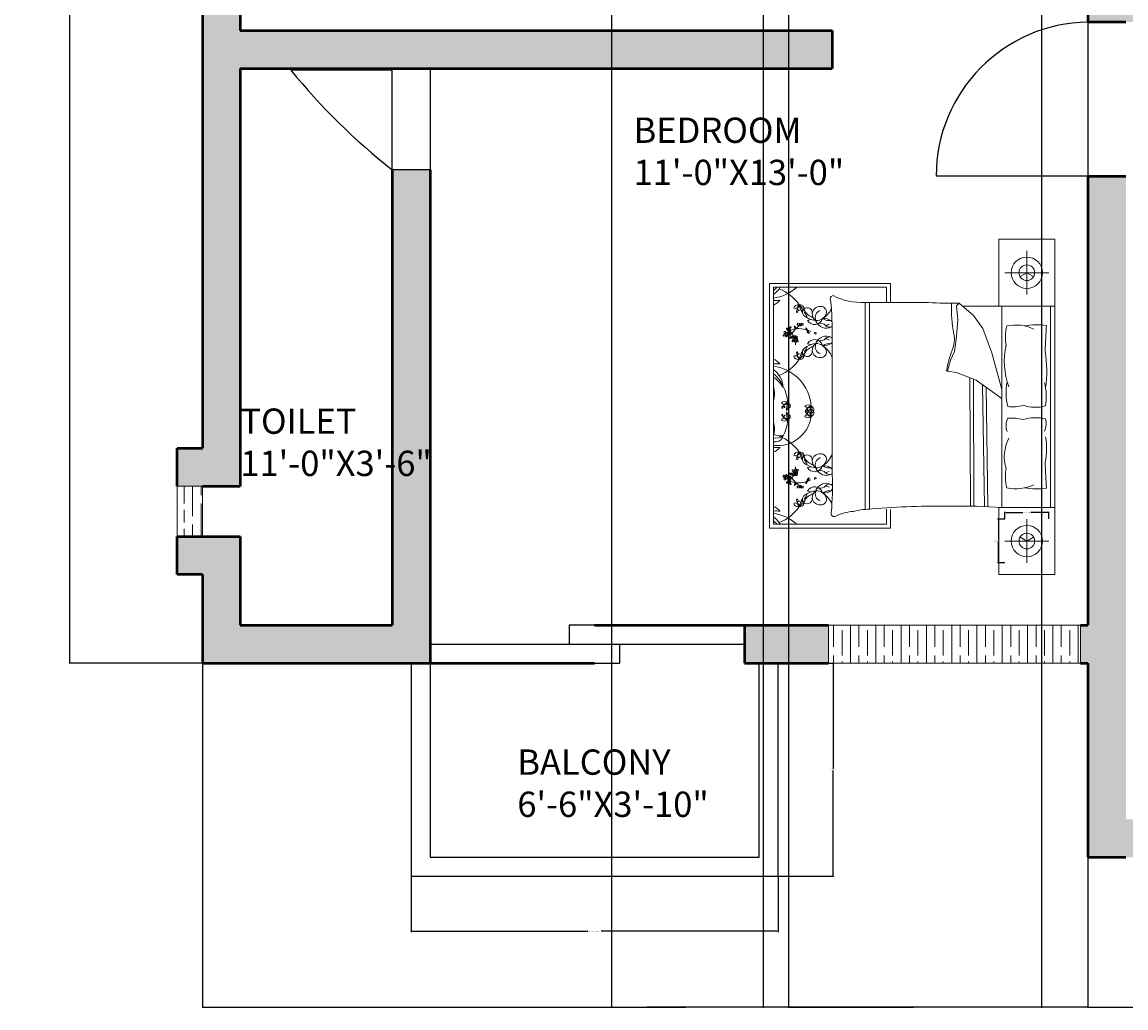
# Model space of a CAD drawing. Units: inches. Extents: x -12 to 604, y -566 to 58.
# Tile 1 of 12: x -12 to 249, y -566 to -332. Entities that reach past the tile are written whole.
import ezdxf

# ---------------------------------------------------------------- set-up
doc = ezdxf.new("R2010")
doc.units = ezdxf.units.IN
doc.header["$MEASUREMENT"] = 0
for name, color, linetype, lineweight in [('A-ANNO-DIMS', 2, 'Continuous', 18), ('A-AREA-IDEN', 7, 'Continuous', 18), ('A-DOOR', 4, 'Continuous', 25), ('A-FLOR-RAIL', 7, 'Continuous', 25), ('A-FURN', 8, 'Continuous', 18), ('A-GLAZ', 82, 'Continuous', 18), ('A-GLAZ-PATT', 82, 'Continuous', 13), ('A-WALL', 7, 'Continuous', 50), ('A-WALL-PATT', 18, 'Continuous', 13)]:
    doc.layers.add(name, color=color, linetype=linetype, lineweight=lineweight)
doc.styles.get("Standard").update_dxf_attribs({"font": 'arial.ttf'})
doc.dimstyles.get("Standard").update_dxf_attribs({"dimtxt": 0.18, "dimasz": 0.18, "dimexe": 0.18, "dimexo": 0.0625, "dimgap": 0.09, "dimtad": 0, "dimtih": 1, "dimtoh": 1, "dimdec": 0, "dimzin": 0, "dimdsep": 46, "dimlunit": 3, "dimtxsty": 'Standard', "dimcen": 0.09, "dimadec": 0, "dimazin": 0, "dimtfac": 1, "dimtdec": 0, "dimtofl": 0, "dimtmove": 0, "dimatfit": 3, "dimfxl": 1, "dimtolj": 1, "dimtzin": 0, "dimarcsym": 0})
pattern_1 = [(90, (0, 0), (6, -4e-16), [10, -2]), (90, (2, -2), (6, -4e-16), [6, -1.5, 3, -1.5]), (90, (4, -5), (6, -4e-16), [10, -2])]

# ---------------------------------------------------------------- blocks, each defined once
blk = doc.blocks.new('*D5')
at = {"layer": 'A-ANNO-DIMS', "color": 0, "lineweight": -2, "transparency": 16777216}
for p, q in [((30.26, 11.14), (-1.3, 11.14)), ((-1.12, 10.96), (-1.12, -233.2)), ((-1.12, -483.68), (-1.12, -239.51)), ((30.26, -483.86), (-1.3, -483.86))]:
    blk.add_line(p, q, dxfattribs=at)
at = {"layer": 'A-ANNO-DIMS', "color": 0, "transparency": 16777216}
for points in [[(-1.15, 10.96), (-1.09, 10.96), (-1.12, 11.14)], [(-1.15, -483.68), (-1.09, -483.68), (-1.12, -483.86)]]:
    blk.add_solid(points, dxfattribs=at)
at = {"layer": 'Defpoints', "color": 0, "transparency": 16777216}
for p in [(30.32, 11.14), (-1.12, -483.86), (30.32, -483.86)]:
    blk.add_point(p, dxfattribs=at)
at = {"layer": 'A-ANNO-DIMS', "color": 0, "transparency": 16777216, "insert": (-1.12, -236.36), "char_height": 6, "attachment_point": 5}
blk.add_mtext('\\A1;41\'-3"', dxfattribs=at)
blk = doc.blocks.new('BALCONY-RAIL-U')
for p, q in [((0, 50.5), (0, 4.5)), ((4.5, 50.5), (4.5, 4.5)), ((82.5, 4.5), (82.5, 50.5)), ((87, 4.5), (87, 50.5)), ((0, 4.5), (0, 0)), ((4.5, 4.5), (82.5, 4.5)), ((87, 0), (87, 4.5)), ((0, 0), (4.5, 0)), ((4.5, 0), (82.5, 0)), ((82.5, 0), (87, 0))]:
    blk.add_line(p, q)
blk = doc.blocks.new('BEDSIDE-LAMP-189')
for p, q in [((5.2, 10.39), (5.2, 0)), ((0, 5.2), (10.39, 5.2))]:
    blk.add_line(p, q)
for points in [[(5.2, 5.2), (3.59, 6.12)], [(5.2, 5.2), (6.8, 6.12)]]:
    blk.add_lwpolyline(points)
for radius in [3.71, 1.86]:
    blk.add_circle((5.2, 5.2), radius)
blk = doc.blocks.new('*D35')
at = {"layer": 'A-ANNO-DIMS', "color": 0, "lineweight": -2, "transparency": 16777216}
for p, q in [((79.82, -534.42), (79.82, -547.59)), ((166.82, -534.42), (166.82, -547.59)), ((80, -547.41), (121.74, -547.41)), ((166.64, -547.41), (124.91, -547.41))]:
    blk.add_line(p, q, dxfattribs=at)
at = {"layer": 'A-ANNO-DIMS', "color": 0, "transparency": 16777216}
for points in [[(80, -547.38), (80, -547.44), (79.82, -547.41)], [(166.64, -547.38), (166.64, -547.44), (166.82, -547.41)]]:
    blk.add_solid(points, dxfattribs=at)
at = {"layer": 'Defpoints', "color": 0, "transparency": 16777216}
for p in [(79.82, -534.36), (166.82, -534.36), (166.82, -547.41)]:
    blk.add_point(p, dxfattribs=at)
at = {"layer": 'A-ANNO-DIMS', "color": 0, "transparency": 16777216, "insert": (123.32, -547.41), "char_height": 0.18, "attachment_point": 5}
blk.add_mtext('\\A1;BALCONY RAIL 7\'-3" TYP.', dxfattribs=at)
blk = doc.blocks.new('*D36')
at = {"layer": 'A-ANNO-DIMS', "color": 0, "lineweight": -2, "transparency": 16777216}
for p, q in [((166.89, -483.86), (180.05, -483.86)), ((179.87, -484.04), (179.87, -508.93)), ((179.87, -534.18), (179.87, -509.29)), ((166.89, -534.36), (180.05, -534.36))]:
    blk.add_line(p, q, dxfattribs=at)
at = {"layer": 'A-ANNO-DIMS', "color": 0, "transparency": 16777216}
for points in [[(179.84, -484.04), (179.9, -484.04), (179.87, -483.86)], [(179.84, -534.18), (179.9, -534.18), (179.87, -534.36)]]:
    blk.add_solid(points, dxfattribs=at)
at = {"layer": 'Defpoints', "color": 0, "transparency": 16777216}
for p in [(166.82, -483.86), (179.87, -483.86), (166.82, -534.36)]:
    blk.add_point(p, dxfattribs=at)
at = {"layer": 'A-ANNO-DIMS', "color": 0, "transparency": 16777216, "insert": (179.87, -509.11), "char_height": 0.18, "attachment_point": 5}
blk.add_mtext('\\A1;4\'-2 1/2" TYP.', dxfattribs=at)
blk = doc.blocks.new('*D45')
at = {"layer": 'A-ANNO-DIMS', "color": 0, "lineweight": -2, "transparency": 16777216}
for p, q in [((220.57, -449.71), (218.89, -449.71)), ((219.07, -449.89), (219.07, -454.72)), ((219.07, -459.92), (219.07, -455.09)), ((220.57, -460.1), (218.89, -460.1))]:
    blk.add_line(p, q, dxfattribs=at)
at = {"layer": 'A-ANNO-DIMS', "color": 0, "transparency": 16777216}
for points in [[(219.04, -449.89), (219.1, -449.89), (219.07, -449.71)], [(219.04, -459.92), (219.1, -459.92), (219.07, -460.1)]]:
    blk.add_solid(points, dxfattribs=at)
at = {"layer": 'Defpoints', "color": 0, "transparency": 16777216}
for p in [(219.07, -449.71), (220.63, -449.71), (220.63, -460.1)]:
    blk.add_point(p, dxfattribs=at)
at = {"layer": 'A-ANNO-DIMS', "color": 0, "transparency": 16777216, "insert": (219.07, -454.91), "char_height": 0.18, "attachment_point": 5}
blk.add_mtext('\\A1;LAMP E 0\'-10 1/2" TYP.', dxfattribs=at)
blk = doc.blocks.new('*D46')
at = {"layer": 'A-ANNO-DIMS', "color": 0, "lineweight": -2, "transparency": 16777216}
for p, q in [((220.63, -449.65), (220.63, -447.97)), ((220.81, -448.15), (224.91, -448.15)), ((230.84, -448.15), (226.74, -448.15)), ((231.02, -449.65), (231.02, -447.97))]:
    blk.add_line(p, q, dxfattribs=at)
at = {"layer": 'A-ANNO-DIMS', "color": 0, "transparency": 16777216}
for points in [[(220.81, -448.12), (220.81, -448.18), (220.63, -448.15)], [(230.84, -448.12), (230.84, -448.18), (231.02, -448.15)]]:
    blk.add_solid(points, dxfattribs=at)
at = {"layer": 'Defpoints', "color": 0, "transparency": 16777216}
for p in [(220.63, -449.71), (231.02, -448.15), (231.02, -449.71)]:
    blk.add_point(p, dxfattribs=at)
at = {"layer": 'A-ANNO-DIMS', "color": 0, "transparency": 16777216, "insert": (225.82, -448.15), "char_height": 0.18, "attachment_point": 5}
blk.add_mtext('\\A1;0\'-10 1/2" TYP.', dxfattribs=at)
blk = doc.blocks.new('*D49')
at = {"layer": 'A-ANNO-DIMS', "color": 0, "lineweight": -2, "transparency": 16777216}
for p, q in [((30.32, -483.92), (30.32, -565.59)), ((240.32, -483.92), (240.32, -565.59)), ((30.5, -565.41), (134.93, -565.41)), ((240.14, -565.41), (135.71, -565.41))]:
    blk.add_line(p, q, dxfattribs=at)
at = {"layer": 'A-ANNO-DIMS', "color": 0, "transparency": 16777216}
for points in [[(30.5, -565.38), (30.5, -565.44), (30.32, -565.41)], [(240.14, -565.38), (240.14, -565.44), (240.32, -565.41)]]:
    blk.add_solid(points, dxfattribs=at)
at = {"layer": 'Defpoints', "color": 0, "transparency": 16777216}
for p in [(30.32, -483.86), (240.32, -483.86), (240.32, -565.41)]:
    blk.add_point(p, dxfattribs=at)
at = {"layer": 'A-ANNO-DIMS', "color": 0, "transparency": 16777216, "insert": (135.32, -565.41), "char_height": 0.18, "attachment_point": 5}
blk.add_mtext('\\A1;17\'-6"', dxfattribs=at)
blk = doc.blocks.new('*D50')
at = {"layer": 'A-ANNO-DIMS', "color": 0, "lineweight": -2, "transparency": 16777216}
for p, q in [((240.32, -529.92), (240.32, -565.59)), ((388.32, -529.92), (388.32, -565.59)), ((240.5, -565.41), (313.93, -565.41)), ((388.14, -565.41), (314.71, -565.41))]:
    blk.add_line(p, q, dxfattribs=at)
at = {"layer": 'A-ANNO-DIMS', "color": 0, "transparency": 16777216}
for points in [[(240.5, -565.38), (240.5, -565.44), (240.32, -565.41)], [(388.14, -565.38), (388.14, -565.44), (388.32, -565.41)]]:
    blk.add_solid(points, dxfattribs=at)
at = {"layer": 'Defpoints', "color": 0, "transparency": 16777216}
for p in [(240.32, -529.86), (388.32, -529.86), (388.32, -565.41)]:
    blk.add_point(p, dxfattribs=at)
at = {"layer": 'A-ANNO-DIMS', "color": 0, "transparency": 16777216, "insert": (314.32, -565.41), "char_height": 0.18, "attachment_point": 5}
blk.add_mtext('\\A1;12\'-4"', dxfattribs=at)
blk = doc.blocks.new('*D56')
at = {"layer": 'A-ANNO-DIMS', "color": 0, "lineweight": -2, "transparency": 16777216}
for p, q in [((127.32, -117.92), (127.32, -565.59)), ((163.32, -117.92), (163.32, -565.59)), ((127.5, -565.41), (144.99, -565.41)), ((163.14, -565.41), (145.65, -565.41))]:
    blk.add_line(p, q, dxfattribs=at)
at = {"layer": 'A-ANNO-DIMS', "color": 0, "transparency": 16777216}
for points in [[(127.5, -565.38), (127.5, -565.44), (127.32, -565.41)], [(163.14, -565.38), (163.14, -565.44), (163.32, -565.41)]]:
    blk.add_solid(points, dxfattribs=at)
at = {"layer": 'Defpoints', "color": 0, "transparency": 16777216}
for p in [(127.32, -117.86), (163.32, -117.86), (163.32, -565.41)]:
    blk.add_point(p, dxfattribs=at)
at = {"layer": 'A-ANNO-DIMS', "color": 0, "transparency": 16777216, "insert": (145.32, -565.41), "char_height": 0.18, "attachment_point": 5}
blk.add_mtext('\\A1;3\'-0"', dxfattribs=at)
blk = doc.blocks.new('*D57')
at = {"layer": 'A-ANNO-DIMS', "color": 0, "lineweight": -2, "transparency": 16777216}
for p, q in [((169.32, 12.58), (169.32, -565.59)), ((229.32, 12.58), (229.32, -565.59)), ((169.5, -565.41), (198.99, -565.41)), ((229.14, -565.41), (199.65, -565.41))]:
    blk.add_line(p, q, dxfattribs=at)
at = {"layer": 'A-ANNO-DIMS', "color": 0, "transparency": 16777216}
for points in [[(169.5, -565.38), (169.5, -565.44), (169.32, -565.41)], [(229.14, -565.38), (229.14, -565.44), (229.32, -565.41)]]:
    blk.add_solid(points, dxfattribs=at)
at = {"layer": 'Defpoints', "color": 0, "transparency": 16777216}
for p in [(169.32, 12.64), (229.32, 12.64), (229.32, -565.41)]:
    blk.add_point(p, dxfattribs=at)
at = {"layer": 'A-ANNO-DIMS', "color": 0, "transparency": 16777216, "insert": (199.32, -565.41), "char_height": 0.18, "attachment_point": 5}
blk.add_mtext('\\A1;5\'-0"', dxfattribs=at)

msp = doc.modelspace()

# ---------------------------------------------------------------- hatches: boundary and pattern name
at = {"layer": 'A-GLAZ-PATT'}
h = msp.add_hatch(dxfattribs=at)
h.set_pattern_fill('GOST_WOOD', color=256)
h.set_pattern_definition(pattern_1)
h.paths.add_polyline_path([(30.32, -441.86), (24.32, -441.86), (24.32, -453.86), (30.32, -453.86)])
h.paths.add_polyline_path([(30.32, -276.86), (24.32, -276.86), (24.32, -318.86), (30.32, -318.86)])
h = msp.add_hatch(dxfattribs=at)
h.set_pattern_fill('GOST_WOOD', color=256)
h.set_pattern_definition(pattern_1)
h.paths.add_polyline_path([(238.52, -474.86), (178.82, -474.86), (178.82, -483.86), (238.52, -483.86)])
at = {"layer": 'A-WALL-PATT'}
h = msp.add_hatch(color=256, dxfattribs=at)
h.dxf.hatch_style = 1
h.paths.add_polyline_path([(169.32, 11.14), (169.32, 17.14), (160.32, 17.14), (160.32, 11.14), (118.32, 11.14), (118.32, 6.64), (118.32, 2.14), (127.32, 2.14), (169.32, 2.14)])
h.paths.add_polyline_path([(127.32, -13.61), (118.32, -13.61), (118.32, -29.36), (34.82, -29.36), (24.32, -29.36), (24.32, -38.36), (39.32, -38.36), (118.32, -38.36), (118.32, -126.86), (127.32, -126.86), (127.32, -117.86)])
h.paths.add_polyline_path([(82.32, -92.36), (39.32, -92.36), (39.32, -56.22), (30.32, -56.22), (24.32, -56.22), (24.32, -65.22), (30.32, -65.22), (30.32, -113.36), (24.32, -113.36), (24.32, -122.36), (39.32, -122.36), (39.32, -101.36), (82.32, -101.36), (82.32, -96.86)], flags=17)
h.paths.add_polyline_path([(280.32, 11.14), (238.32, 11.14), (238.32, 17.14), (229.32, 17.14), (229.32, 12.64), (229.32, 11.14), (229.32, 2.14), (271.32, 2.14), (271.32, -117.86), (163.32, -117.86), (163.32, -126.86), (271.32, -126.86), (271.32, -189.86), (280.32, -189.86), (280.32, -180.86)])
h.paths.add_polyline_path([(415.32, 17.14), (406.32, 17.14), (406.32, 11.14), (358.32, 11.14), (358.32, -21.86), (367.32, -21.86), (367.32, 2.14), (415.32, 2.14)], flags=17)
h.paths.add_polyline_path([(484.55, -45.86), (448.32, -45.86), (448.32, 2.14), (448.32, 17.14), (439.32, 17.14), (439.32, 12.64), (439.32, 2.14), (439.32, -45.86), (367.32, -45.86), (358.32, -45.86), (358.32, -54.86), (430.32, -54.86), (430.32, -69.59), (430.32, -180.86), (318.82, -180.86), (318.82, -189.86), (318.82, -331.86), (327.82, -331.86), (327.82, -189.86), (439.32, -189.86), (439.32, -180.86), (439.32, -54.86), (483.5, -54.86), (484.55, -54.86)])
h.paths.add_polyline_path([(529.32, 11.14), (481.32, 11.14), (481.32, 17.14), (472.32, 17.14), (472.32, 12.64), (472.32, 2.14), (520.32, 2.14), (520.32, -21.86), (529.32, -21.86)])
h.paths.add_polyline_path([(598.32, -45.86), (582.42, -45.86), (582.42, -50.36), (582.42, -54.86), (589.32, -54.86), (589.32, -99.86), (598.32, -99.86), (604.32, -99.86), (604.32, -90.86), (598.32, -90.86)])
h.paths.add_polyline_path([(598.32, -168.86), (604.32, -168.86), (604.32, -159.86), (589.32, -159.86), (589.32, -180.86), (477.32, -180.86), (477.32, -189.86), (477.32, -259.86), (486.32, -259.86), (486.32, -189.86), (589.32, -189.86), (589.32, -204.86), (598.32, -204.86), (604.32, -204.86), (604.32, -195.86), (598.32, -195.86)])
h.paths.add_polyline_path([(598.32, -244.86), (604.32, -244.86), (604.32, -235.86), (598.32, -235.86), (589.32, -235.86), (589.32, -250.86), (522.32, -250.86), (522.32, -259.86), (589.32, -259.86), (589.32, -274.86), (598.32, -274.86), (604.32, -274.86), (604.32, -265.86), (598.32, -265.86)])
h.paths.add_polyline_path([(598.32, -333.28), (604.32, -333.28), (604.32, -324.28), (598.32, -324.28), (598.32, -321.87), (598.32, -318.28), (604.32, -318.28), (604.32, -309.28), (598.32, -309.28), (589.32, -309.28), (589.32, -341.95), (589.38, -341.95), (589.38, -363.16), (589.32, -381.86), (565.32, -381.86), (565.32, -390.86), (589.32, -390.86), (589.32, -450.86), (598.32, -450.86), (604.32, -450.86), (604.32, -441.86), (598.32, -441.86), (598.32, -390.86), (604.32, -390.86), (604.32, -381.86), (598.32, -381.86)])
h.paths.add_polyline_path([(541.32, -345.86), (424.32, -345.86), (424.32, -354.86), (532.32, -354.86), (532.32, -474.86), (463.39, -474.86), (463.39, -483.86), (553.32, -483.86), (553.32, -474.86), (541.32, -474.86), (541.32, -390.86), (541.32, -381.86)])
h.paths.add_polyline_path([(604.32, -474.86), (589.32, -474.86), (553.32, -474.86), (553.32, -483.86), (598.32, -483.86), (604.32, -483.86)])
h.paths.add_polyline_path([(388.32, -483.86), (388.32, -474.86), (388.32, -460.13), (388.32, -333.86), (388.32, -322.86), (379.32, -322.86), (379.32, -331.86), (379.32, -333.86), (379.32, -474.86), (379.32, -520.86), (344.32, -520.86), (344.32, -529.86), (379.32, -529.86), (388.32, -529.86)])
h.paths.add_polyline_path([(284.32, -520.86), (249.32, -520.86), (249.32, -474.86), (249.32, -368.36), (240.32, -368.36), (240.32, -474.86), (238.52, -474.86), (238.52, -483.86), (240.32, -483.86), (240.32, -529.86), (249.32, -529.86), (284.32, -529.86)])
h.paths.add_polyline_path([(178.82, -474.86), (158.91, -474.86), (158.91, -483.86), (162.32, -483.86), (178.82, -483.86)])
h.paths.add_polyline_path([(84.32, -474.86), (84.32, -366.86), (75.32, -366.86), (75.32, -474.86), (39.32, -474.86), (39.32, -453.86), (24.32, -453.86), (24.32, -462.86), (30.32, -462.86), (30.32, -483.86), (84.32, -483.86)])
h.paths.add_polyline_path([(39.32, -342.86), (75.32, -342.86), (84.32, -342.86), (179.67, -342.86), (179.67, -333.86), (39.32, -333.86), (39.32, -318.86), (24.32, -318.86), (24.32, -327.86), (30.32, -327.86), (30.32, -432.86), (24.32, -432.86), (24.32, -441.86), (30.32, -441.86), (39.32, -441.86)])
h.paths.add_polyline_path([(249.32, -252.86), (115.32, -252.86), (115.32, -225.86), (106.32, -225.86), (106.32, -252.86), (39.32, -252.86), (39.32, -237.86), (24.32, -237.86), (24.32, -246.86), (30.32, -246.86), (30.32, -267.86), (24.32, -267.86), (24.32, -276.86), (39.32, -276.86), (39.32, -261.86), (240.32, -261.86), (240.32, -331.86), (249.32, -331.86), (266.82, -331.86), (266.82, -322.86), (249.32, -322.86)])
h.paths.add_polyline_path([(127.32, -180.86), (39.32, -180.86), (24.32, -180.86), (24.32, -189.86), (39.32, -189.86), (127.32, -189.86)])
h.paths.add_polyline_path([(39.32, -159.86), (24.32, -159.86), (24.32, -168.86), (30.32, -168.86), (30.32, -180.86), (39.32, -180.86)])
h.paths.add_polyline_path([(470.51, -17.27), (512.48, -17.27), (512.48, 5.12), (470.51, 5.12)], flags=9)
h.paths.add_polyline_path([(484.21, -244.26), (526.45, -244.26), (526.45, -221.87), (484.21, -221.87)], flags=24)
h.paths.add_polyline_path([(36.91, -442.88), (83.54, -442.88), (83.54, -420.5), (36.91, -420.5)], flags=25)

# ---------------------------------------------------------------- linework, layer by layer
at = {"layer": 'A-DOOR'}
for p, q in [((240.32, -331.86), (240.32, -368.36)), ((84.32, -342.86), (75.32, -342.86)), ((75.32, -366.86), (75.32, -342.86)), ((84.32, -342.86), (84.32, -366.86)), ((75.32, -343.26), (51.32, -343.26)), ((84.32, -366.86), (75.32, -366.86)), ((240.32, -368.36), (204.32, -368.36)), ((123.32, -474.86), (117.32, -474.86)), ((117.32, -474.86), (117.32, -479.36)), ((84.32, -479.36), (158.91, -479.36)), ((129.32, -483.86), (129.32, -479.36)), ((123.32, -483.86), (129.32, -483.86))]:
    msp.add_line(p, q, dxfattribs=at)
for centre, radius, start, end in [((240.83, -368.36), 36.5, 90.7903, 180), ((167.54, -249.09), 149.57, 219.0162, 231.9382)]:
    msp.add_arc(centre, radius, start, end, dxfattribs=at)
at = {"layer": 'A-FURN'}
for p, q in [((232.45, -383.32), (232.45, -462.86)), ((164.81, -393.82), (193.46, -393.82)), ((164.81, -451.81), (164.81, -393.82)), ((165.73, -394.74), (165.73, -450.88)), ((192.54, -394.74), (165.73, -394.74)), ((192.54, -398.31), (192.54, -394.74)), ((193.46, -393.82), (193.46, -398.32)), ((187.51, -447.39), (187.51, -398.31)), ((188.5, -447.31), (188.5, -398.31)), ((209.15, -399.16), (209.79, -398.51)), ((209.47, -402.38), (209.15, -399.16)), ((209.79, -398.51), (213.17, -401.41)), ((232.45, -399.23), (210.62, -399.23)), ((219.88, -399.23), (219.88, -446.95)), ((231.43, -446.95), (231.43, -399.23)), ((173.79, -402.58), (174.69, -402.4)), ((209.15, -406.41), (209.47, -402.38)), ((213.17, -401.41), (215.43, -404.48)), ((215.43, -404.48), (217.52, -410.28)), ((173.79, -408.14), (174.69, -408.31)), ((179.7, -439.24), (179.7, -406.94)), ((208.66, -409.95), (209.15, -406.41)), ((207.7, -412.05), (208.66, -409.95)), ((217.52, -410.28), (219.88, -418.95)), ((207.05, -414.63), (207.7, -412.05)), ((209.15, -414.95), (207.05, -414.63)), ((213.82, -416.72), (209.15, -414.95)), ((212.44, -446.67), (212.32, -416.15)), ((213.26, -446.67), (213.14, -416.46)), ((219.88, -421.08), (213.82, -416.72)), ((215.76, -446.71), (215.35, -417.83)), ((216.58, -446.74), (216.18, -418.42)), ((173.79, -437.49), (174.69, -437.31)), ((173.79, -443.05), (174.69, -443.22)), ((192.54, -450.88), (192.54, -447.38)), ((193.46, -447.4), (193.46, -451.81)), ((193.46, -451.81), (164.81, -451.81)), ((165.73, -450.88), (192.54, -450.88))]:
    msp.add_line(p, q, dxfattribs=at)
for points in [[(219.2, -399.23), (219.2, -383.32), (232.45, -383.32)], [(232.45, -446.95), (219.2, -446.95), (219.2, -462.86), (232.45, -462.86)]]:
    msp.add_lwpolyline(points, dxfattribs=at)
for points in [[(202.51, -398.35, 0.001242), (187.42, -398.31, -0.127202), (179.89, -396.72)], [(230.47, -403.8, 0.074897), (225.28, -403.89, -0.472817)], [(224.98, -422.72, 0.14099), (230.28, -422.88, 0.235245)], [(224.98, -426.11, -0.14099), (230.28, -425.95, -0.235245)], [(230.47, -442.38, -0.074897), (225.28, -442.29, 0.472817)], [(189.13, -447.29, 0.056112), (184.75, -447.87, 0.095341), (180.54, -448.99)]]:
    msp.add_lwpolyline(points, format="xyb", dxfattribs=at)
for centre in [(168.78, -405.85), (170.91, -407.17), (168.78, -439.78), (170.91, -438.45)]:
    msp.add_circle(centre, 0.203, dxfattribs=at)
for centre, radius, start, end in [((162, -390.4), 6.31, 306.3036, 316.4814), ((162.94, -392.22), 5.06, 303.4617, 330.1116), ((164.33, -387.01), 10.39, 277.745, 311.8856), ((163.3, -404.78), 10.39, 34.3865, 68.5908), ((164.11, -395.05), 4.22, 292.5547, 318.9546), ((166.38, -383.48), 14.37, 267.4081, 273.6519), ((179.94, -397.45), 0.734, 93.98, 207.3412), ((96.9, -405.99), 82.8, 359.3433, 5.6887), ((171.63, -400.04), 1.15, 77.7115, 159.0387), ((171.01, -398.88), 0.867, 238.4633, 358.2869), ((173.85, -400.64), 2.63, 138.8402, 177.9352), ((171.42, -400.54), 0.0627, 11.4834, 127.9409), ((172.27, -399.66), 0.85, 117.6827, 223.7762), ((171.74, -400.17), 0.112, 223.7762, 159.7183), ((172.08, -399.75), 0.861, 2.9516, 103.728), ((178.97, -397.34), 7.27, 192.5173, 207.1824), ((170.92, -400.24), 1.64, 345.4653, 54.2343), ((173.39, -397.99), 1.77, 211.3827, 255.2969), ((173.73, -400.76), 1.19, 350.264, 160.8688), ((174.09, -400.47), 1.49, 175.969, 254.3045), ((172.44, -400.51), 0.732, 333.9755, 53.2681), ((176.36, -398.39), 3.76, 211.2614, 251.7045), ((176.79, -401.2), 1.9, 84.9449, 172.8857), ((177.51, -401.94), 1.85, 111.5819, 201.4221), ((176.98, -400.64), 1.34, 354.4856, 91.0538), ((174.09, -397.14), 6.02, 303.6671, 333.2997), ((207.81, -325.58), 72.96, 265.8294, 271.553), ((237.96, -399.88), 30.02, 177.4519, 191.3392), ((171.36, -400.55), 0.129, 177.9352, 11.4834), ((172.11, -402.08), 1.59, 6.1662, 51.5825), ((176.05, -398.36), 4.27, 236.2883, 266.5076), ((175.51, -401.59), 1.98, 209.9085, 343.1337), ((177.21, -400.86), 2.31, 182.3591, 234.0401), ((175.99, -400.23), 2.39, 265.2933, 346.921), ((176.34, -402.84), 0.494, 167.3041, 285.1471), ((177.68, -405.21), 3.07, 122.7011, 126.3445), ((178.25, -401.9), 2.53, 199.2822, 299.1751), ((179.11, -399.35), 3.3, 238.8218, 279.1554), ((177.68, -405.21), 3.07, 55.785, 94.7304), ((178.82, -403.43), 0.958, 30.0293, 52.325), ((168.62, -405.44), 0.4, 157.4086, 261.4386), ((168.4, -405.42), 0.201, 58.0499, 135.6268), ((168.61, -405.55), 0.134, 172.906, 277.132), ((168.16, -405.79), 0.639, 14.7558, 58.0499), ((169.06, -405.62), 0.276, 36.1046, 181.4281), ((169.07, -404.54), 0.226, 124.3538, 214.3923), ((169.4, -404.57), 0.527, 190.3057, 287.1958), ((168.9, -405.41), 0.279, 270.0645, 331.1507), ((169.14, -405.47), 0.319, 221.8413, 265.7877), ((169.56, -404.39), 0.612, 176.9701, 248.2913), ((173.93, -401.16), 5.92, 212.6784, 216.3746), ((169.13, -405.59), 0.198, 263.7526, 41.7054), ((169.35, -404.53), 0.234, 216.3746, 291.7548), ((171.42, -407.82), 3.3, 124.0033, 132.4917), ((168.02, -408.23), 3.53, 63.7819, 68.2913), ((169.91, -405.52), 0.561, 128.3208, 208.8162), ((169.91, -404.69), 0.527, 122.8155, 187.3992), ((169.5, -404.91), 0.177, 289.3605, 111.7548), ((169.63, -404.91), 0.177, 221.8703, 44.2646), ((170.43, -405.43), 0.923, 157.2305, 229.0635), ((170.14, -404.76), 0.612, 109.4799, 177.6828), ((170.12, -405.12), 0.543, 174.4544, 220.6188), ((167.03, -408.16), 3.96, 30.544, 49.818), ((169.81, -404.37), 0.226, 56.8636, 146.9021), ((169.93, -404.63), 0.234, 148.8844, 224.2646), ((169.22, -405.9), 0.653, 340.0041, 40.6188), ((174.79, -407.56), 5.92, 145.1882, 148.8844), ((171.42, -407.82), 3.3, 94.756, 119.2041), ((178.45, -412.57), 10.87, 132.2412, 142.1744), ((172.97, -403.92), 2.24, 178.3264, 187.1302), ((170.54, -404.23), 0.418, 11.3256, 64.4621), ((171.96, -403.63), 1.26, 190.2588, 210.656), ((171.12, -404.14), 0.382, 188.3432, 274.2869), ((171.45, -403.93), 0.667, 210.656, 242.6341), ((171.96, -403.36), 1.28, 218.2101, 226.3071), ((171.01, -404.43), 0.162, 325.7657, 67.4417), ((165.98, -399.02), 7.55, 313.1541, 322.0459), ((171.59, -411.1), 6.59, 73.5842, 93.8277), ((171.54, -403.55), 0.155, 142.4737, 265.053), ((171.74, -403.52), 0.334, 127.7621, 169.0403), ((171.56, -403.24), 0.471, 265.053, 338.3618), ((172.19, -403.88), 0.615, 113.4276, 137.6104), ((172.12, -403.25), 0.203, 183.2768, 356.7232), ((172.26, -403.61), 0.331, 139.7889, 227.6792), ((172.16, -403.73), 0.175, 227.6792, 350.3487), ((171.48, -403.61), 0.663, 353.0852, 15.7171), ((171.92, -403.69), 0.419, 350.3487, 43.6538), ((172.69, -403.25), 0.487, 198.7263, 262.5032), ((172.31, -403.48), 0.193, 1.1081, 91.8675), ((172.43, -403.53), 0.338, 11.5637, 52.6358), ((172.67, -403.59), 0.157, 255.2356, 54.9248), ((175.64, -404.4), 2.24, 178.3264, 187.1302), ((173.22, -404.71), 0.418, 11.3256, 64.4621), ((174.64, -404.11), 1.26, 190.2588, 210.656), ((173.8, -404.62), 0.382, 188.3432, 274.2869), ((174.13, -404.41), 0.667, 210.656, 242.6341), ((174.63, -403.83), 1.28, 218.2101, 226.3071), ((173.69, -404.91), 0.162, 325.7657, 67.4417), ((174.15, -405.2), 0.382, 147.5332, 233.4768), ((174.49, -405.01), 0.667, 179.1859, 211.164), ((173.84, -405.16), 0.162, 354.3784, 96.0543), ((171.59, -411.1), 6.59, 63.0032, 69.8941), ((175, -404.7), 1.26, 211.164, 231.5612), ((175.22, -403.68), 2.24, 234.6898, 243.4936), ((175.23, -404.83), 1.28, 195.5129, 203.6099), ((173.8, -405.67), 0.418, 357.3579, 50.4944), ((175.59, -405.59), 0.153, 12.7051, 190.4384), ((175.69, -405.57), 0.249, 190.4384, 10.4136), ((176.89, -404.89), 1.63, 41.5653, 105.1471), ((177.79, -401.52), 2.29, 277.436, 299.9149), ((179.01, -403.02), 1.19, 221.5653, 293.8354), ((178.82, -403.43), 0.958, 314.4517, 333.558), ((231.4, -406.63), 10.66, 165.1039, 191.0369), ((223.19, -413.93), 10.25, 65.1316, 101.7583), ((987.44, -447.64), 758.24, 176.68521, 177.14978), ((168.2, -406.15), 0.155, 142.4737, 265.053), ((168.4, -406.12), 0.334, 61.2196, 169.0403), ((168.22, -405.84), 0.471, 265.053, 338.3618), ((168.85, -406.48), 0.615, 113.4276, 137.6104), ((168.93, -406.21), 0.331, 139.7889, 227.6792), ((168.82, -406.33), 0.175, 227.6792, 350.3487), ((168.14, -406.21), 0.663, 353.0852, 15.7171), ((168.58, -406.29), 0.419, 350.3487, 43.6538), ((169.36, -405.86), 0.487, 198.7263, 262.5032), ((168.97, -406.08), 0.193, 1.1081, 91.8675), ((169.09, -406.13), 0.338, 11.5637, 86.365), ((169.33, -406.19), 0.157, 255.2356, 54.9248), ((170.01, -405.48), 0.671, 207.7043, 254.3516), ((169.57, -405.86), 0.923, 270.278, 342.111), ((170.19, -407.02), 0.653, 98.7227, 159.3375), ((169.86, -406.18), 0.671, 244.9899, 291.6373), ((170.01, -405.83), 0.543, 278.7227, 324.8872), ((169.91, -406.28), 0.561, 290.5253, 358.5375), ((170.33, -407.48), 0.155, 142.4737, 265.053), ((170.54, -407.45), 0.334, 61.2196, 169.0403), ((170.36, -407.17), 0.471, 265.053, 338.3618), ((170.76, -406.76), 0.4, 157.4086, 261.4386), ((170.53, -406.75), 0.201, 58.0499, 135.6268), ((171.01, -406.12), 0.561, 182.8499, 266.1226), ((170.79, -405.72), 0.543, 231.7607, 277.9252), ((171.21, -405.62), 0.923, 214.5369, 286.3699), ((170.98, -407.81), 0.615, 113.4276, 137.6104), ((170.74, -406.87), 0.134, 172.906, 277.132), ((170.3, -407.12), 0.639, 14.7558, 58.0499), ((167.03, -408.16), 3.96, 23.0501, 23.8477), ((171.06, -407.54), 0.331, 139.7889, 227.6792), ((170.96, -407.66), 0.175, 227.6792, 350.3487), ((170.95, -406.9), 0.653, 37.3105, 97.9252), ((171.19, -406.95), 0.276, 36.1046, 181.4281), ((170.28, -407.53), 0.663, 353.0852, 15.7171), ((171.03, -406.01), 0.671, 265.0106, 311.658), ((167.03, -408.16), 3.96, 357.1071, 4.7585), ((170.71, -407.61), 0.419, 350.3487, 43.6538), ((171.03, -406.73), 0.279, 270.0645, 331.1507), ((171.27, -406.8), 0.319, 221.8413, 265.7877), ((171.49, -407.18), 0.487, 198.7263, 262.5032), ((171.1, -407.41), 0.193, 1.1081, 91.8675), ((171.27, -406.92), 0.198, 263.7526, 41.7054), ((171.23, -407.45), 0.338, 11.5637, 86.365), ((171.47, -407.51), 0.157, 255.2356, 54.9248), ((176.05, -412.36), 4.27, 93.4924, 123.7117), ((175.51, -409.12), 1.98, 16.8663, 150.0915), ((177.21, -409.85), 2.31, 125.9599, 177.6409), ((177.51, -408.77), 1.85, 158.5779, 248.4181), ((175.99, -410.48), 2.39, 13.079, 94.7067), ((176.34, -407.87), 0.494, 74.8529, 192.6959), ((178.25, -408.82), 2.53, 60.8249, 160.7178), ((177.68, -405.51), 3.07, 233.6555, 237.2989), ((176.89, -405.82), 1.63, 254.8529, 318.4347), ((179.11, -411.37), 3.3, 79.7133, 121.1782), ((177.68, -405.51), 3.07, 265.2696, 304.215), ((177.79, -409.2), 2.29, 60.0851, 82.564), ((179.01, -407.69), 1.19, 66.1646, 138.4347), ((178.82, -407.29), 0.958, 307.675, 336.7144), ((178.82, -407.29), 0.958, 23.229, 45.5483), ((202.18, -407.05), 6.47, 336.2616, 11.3392), ((171.36, -410.16), 0.129, 348.5166, 182.0648), ((173.85, -410.07), 2.63, 182.0648, 221.1598), ((171.42, -410.18), 0.0627, 232.0591, 348.5166), ((172.27, -411.05), 0.85, 136.2238, 242.3173), ((171.78, -410.55), 0.0677, 200.2667, 136.2271), ((170.92, -410.47), 1.64, 305.7657, 14.5347), ((178.97, -413.38), 7.27, 152.8176, 167.4827), ((174.09, -410.24), 1.49, 105.6955, 184.031), ((173.73, -409.96), 1.19, 199.1312, 9.736), ((172.44, -410.2), 0.732, 306.7319, 26.0245), ((172.11, -408.64), 1.59, 308.4175, 353.8338), ((176.36, -412.32), 3.76, 108.2955, 148.7386), ((176.79, -409.52), 1.9, 187.1143, 275.0551), ((176.98, -410.07), 1.34, 268.9462, 5.5144), ((174.09, -413.58), 6.02, 21.4941, 56.3329), ((237.11, -420.15), 30.85, 160.1194, 169.3383), ((238.98, -412.24), 18.49, 168.0397, 199.2615), ((201.69, -414.69), 28.85, 352.2196, 9.497), ((164.11, -415.66), 4.22, 41.0454, 67.4453), ((166.38, -427.23), 14.37, 86.3481, 92.5919), ((164.33, -423.71), 10.39, 4.4623, 82.255), ((163.3, -405.94), 10.39, 291.4092, 325.6135), ((171.01, -411.83), 0.867, 1.7131, 121.5367), ((171.63, -410.68), 1.15, 200.9613, 282.2885), ((172.08, -410.97), 0.861, 256.272, 357.0484), ((173.39, -412.73), 1.77, 104.7031, 148.6173), ((162.94, -418.5), 5.06, 1.272, 56.5383), ((162, -420.32), 6.31, 17.8504, 53.6964), ((160.22, -423.63), 9.38, 34.0123, 54.053), ((206.99, -414.44), 0.192, 178.8623, 289.7536), ((160.27, -420.01), 5.71, 343.5431, 17.0202), ((158.77, -422.91), 10.39, 4.4623, 27.4146), ((234.94, -419.73), 14.03, 169.8617, 193.6238), ((216.27, -420.79), 14.17, 351.5249, 13.96), ((157.33, -422.27), 8.45, 4.3787, 5.6357), ((151.54, -426.72), 15.09, 19.7217, 19.9028), ((168.35, -422.96), 1.15, 47.7873, 129.1145), ((168.38, -421.65), 0.867, 208.5391, 328.3627), ((167.86, -423.27), 0.129, 148.011, 341.5592), ((169.97, -424.59), 2.63, 108.9159, 148.011), ((167.92, -423.29), 0.0627, 341.5592, 98.0167), ((169.09, -422.95), 0.85, 87.7585, 193.852), ((168.37, -423.13), 0.112, 193.852, 129.9245), ((176.06, -424.28), 7.27, 162.593, 177.2582), ((167.63, -422.78), 1.64, 315.5411, 24.3101), ((170.9, -422.06), 1.77, 181.4585, 225.3727), ((168.88, -422.93), 0.861, 333.0274, 73.8037), ((173.91, -423.75), 1.15, 47.7873, 129.1145), ((173.95, -422.44), 0.867, 208.5391, 328.3627), ((173.42, -424.06), 0.129, 148.011, 341.5592), ((175.54, -425.38), 2.63, 108.9159, 148.011), ((173.48, -424.08), 0.0627, 341.5592, 98.0167), ((174.65, -423.75), 0.85, 87.7585, 193.852), ((173.94, -423.93), 0.112, 193.852, 129.9245), ((173.19, -423.58), 1.64, 315.5411, 24.3101), ((181.62, -425.07), 7.27, 162.593, 177.2582), ((173.19, -424.7), 1.64, 335.6899, 44.4589), ((181.62, -423.2), 7.27, 182.7418, 197.407), ((174.45, -423.73), 0.861, 333.0274, 73.8037), ((176.46, -422.85), 1.77, 181.4585, 225.3727), ((222.33, -413.34), 9.75, 264.0129, 285.8293), ((166.73, -424.23), 8.04, 262.8636, 351.8197), ((160.27, -428.27), 5.71, 342.9798, 16.4569), ((157.33, -426), 8.45, 354.3643, 355.6213), ((151.54, -421.56), 15.09, 340.0972, 340.2783), ((168.38, -426.63), 0.867, 31.6373, 151.4609), ((168.35, -425.32), 1.15, 230.8855, 312.2127), ((167.86, -425.01), 0.129, 18.4408, 211.989), ((169.97, -423.69), 2.63, 211.989, 251.0841), ((167.92, -424.99), 0.0627, 261.9833, 18.4408), ((158.77, -425.36), 10.39, 332.5854, 355.5377), ((169.09, -425.32), 0.85, 166.148, 272.2415), ((168.42, -425.13), 0.0677, 230.1909, 166.0209), ((176.06, -424), 7.27, 182.7418, 197.407), ((167.63, -425.49), 1.64, 335.6899, 44.4589), ((170.9, -426.22), 1.77, 134.6273, 178.5415), ((168.88, -425.34), 0.861, 286.1963, 26.9726), ((173.95, -425.83), 0.867, 31.6373, 151.4609), ((173.91, -424.52), 1.15, 230.8855, 312.2127), ((173.42, -424.21), 0.129, 18.4408, 211.989), ((175.54, -422.89), 2.63, 211.989, 251.0841), ((173.48, -424.19), 0.0627, 261.9833, 18.4408), ((174.65, -424.53), 0.85, 166.148, 272.2415), ((173.98, -424.34), 0.0677, 230.1909, 166.0209), ((174.45, -424.55), 0.861, 286.1963, 26.9726), ((176.46, -425.42), 1.77, 134.6273, 178.5415), ((225.13, -427.58), 4.22, 155.0183, 198.5407), ((222.33, -435.49), 9.75, 74.1707, 95.9871), ((226.5, -427.05), 3.93, 333.3437, 16.1026), ((167.46, -425.27), 4.65, 248.117, 276.6195), ((166.17, -429.54), 1.86, 256.3898, 349.0739), ((166.42, -428.14), 2.36, 252.8609, 311.9049), ((163.3, -439.69), 10.39, 34.3865, 68.5908), ((230.62, -434.95), 10.13, 153.8761, 196.1746), ((216.55, -432.94), 13.98, 346.3427, 11.1841), ((166.38, -418.39), 14.37, 267.4081, 273.6519), ((164.11, -429.96), 4.22, 292.5547, 318.9546), ((171.63, -434.95), 1.15, 77.7115, 159.0387), ((171.01, -433.79), 0.867, 238.4633, 358.2869), ((173.85, -435.55), 2.63, 138.8402, 177.9352), ((172.27, -434.57), 0.85, 117.6827, 223.7762), ((172.08, -434.66), 0.861, 2.9516, 103.728), ((173.39, -432.9), 1.77, 211.3827, 255.2969), ((170.92, -435.15), 1.64, 345.4653, 54.2343), ((178.97, -432.25), 7.27, 192.5173, 207.1824), ((173.73, -435.67), 1.19, 350.264, 160.8688), ((176.79, -436.11), 1.9, 84.9449, 172.8857), ((176.98, -435.55), 1.34, 354.4856, 91.0538), ((174.09, -432.05), 6.02, 303.6671, 338.5059), ((171.36, -435.46), 0.129, 177.9352, 11.4834), ((171.42, -435.45), 0.0627, 11.4834, 127.9409), ((171.74, -435.08), 0.112, 223.7762, 159.7183), ((174.09, -435.38), 1.49, 175.969, 254.3045), ((172.44, -435.42), 0.732, 333.9755, 53.2681), ((172.11, -436.99), 1.59, 6.1662, 51.5825), ((176.36, -433.3), 3.76, 211.2614, 251.7045), ((176.05, -433.27), 4.27, 236.2883, 266.5076), ((175.51, -436.5), 1.98, 209.9085, 343.1337), ((177.21, -435.77), 2.31, 182.3591, 234.0401), ((177.51, -436.85), 1.85, 111.5819, 201.4221), ((175.99, -435.14), 2.39, 265.2933, 346.921), ((179.11, -434.26), 3.3, 238.8218, 280.2867), ((177.68, -440.12), 3.07, 55.785, 94.7304), ((987.44, -398.54), 758.24, 182.85022, 183.31479), ((168.2, -439.47), 0.155, 94.947, 217.5263), ((168.4, -439.5), 0.334, 190.9597, 298.7804), ((168.22, -439.78), 0.471, 21.6382, 94.947), ((168.85, -439.14), 0.615, 222.3896, 246.5724), ((168.93, -439.41), 0.331, 132.3208, 220.2111), ((168.82, -439.29), 0.175, 9.6513, 132.3208), ((168.14, -439.41), 0.663, 344.2829, 6.9148), ((168.58, -439.33), 0.419, 316.3462, 9.6513), ((169.36, -439.77), 0.487, 97.4968, 161.2737), ((168.97, -439.54), 0.193, 268.1325, 358.8919), ((169.09, -439.5), 0.338, 273.635, 348.4363), ((169.33, -439.44), 0.157, 305.0752, 104.7644), ((170.01, -440.15), 0.671, 105.6484, 152.2957), ((170.43, -440.2), 0.923, 130.9365, 202.7695), ((169.86, -439.45), 0.671, 68.3627, 115.0101), ((169.57, -439.76), 0.923, 17.889, 89.722), ((170.19, -438.61), 0.653, 200.6625, 261.2773), ((167.03, -437.47), 3.96, 310.182, 329.456), ((169.22, -439.72), 0.653, 319.3812, 19.9959), ((178.45, -433.05), 10.87, 217.8256, 227.7588), ((170.01, -439.79), 0.543, 35.1128, 81.2773), ((169.91, -439.35), 0.561, 1.4625, 69.4747), ((170.33, -438.14), 0.155, 94.947, 217.5263), ((170.54, -438.17), 0.334, 190.9597, 298.7804), ((170.36, -438.46), 0.471, 21.6382, 94.947), ((170.76, -438.86), 0.4, 98.5614, 202.5914), ((170.53, -438.88), 0.201, 224.3732, 301.9501), ((171.01, -439.51), 0.561, 93.8774, 177.1501), ((171.21, -440), 0.923, 73.6301, 145.4631), ((170.79, -439.9), 0.543, 82.0748, 128.2393), ((170.98, -437.81), 0.615, 222.3896, 246.5724), ((170.74, -438.75), 0.134, 82.868, 187.094), ((170.3, -438.5), 0.639, 301.9501, 345.2442), ((167.03, -437.47), 3.96, 336.1523, 336.9499), ((171.06, -438.08), 0.331, 132.3208, 220.2111), ((170.96, -437.97), 0.175, 9.6513, 132.3208), ((170.95, -438.72), 0.653, 262.0748, 322.6895), ((170.28, -438.09), 0.663, 344.2829, 6.9148), ((171.19, -438.67), 0.276, 178.5719, 323.8954), ((171.03, -439.62), 0.671, 48.342, 94.9894), ((167.03, -437.47), 3.96, 355.2415, 2.8929), ((170.71, -438.01), 0.419, 316.3462, 9.6513), ((171.49, -438.44), 0.487, 97.4968, 161.2737), ((171.27, -438.83), 0.319, 94.2123, 138.1587), ((171.03, -438.89), 0.279, 28.8493, 89.9355), ((171.1, -438.21), 0.193, 268.1325, 358.8919), ((171.23, -438.17), 0.338, 273.635, 348.4363), ((171.27, -438.71), 0.198, 318.2946, 96.2474), ((171.47, -438.11), 0.157, 305.0752, 104.7644), ((176.34, -437.75), 0.494, 167.3041, 285.1471), ((177.68, -440.12), 3.07, 122.7011, 126.3445), ((178.25, -436.81), 2.53, 199.2822, 299.1751), ((176.89, -439.8), 1.63, 41.5653, 105.1471), ((177.79, -436.43), 2.29, 277.436, 299.9149), ((179.01, -437.93), 1.19, 221.5653, 293.8354), ((178.82, -438.34), 0.958, 23.2856, 52.325), ((102.33, -441.67), 77.4, 355.2402, 1.8035), ((178.82, -438.34), 0.958, 314.4517, 336.7144), ((231.4, -439.55), 10.66, 168.9631, 194.8961), ((168.62, -440.19), 0.4, 98.5614, 202.5914), ((168.4, -440.2), 0.201, 224.3732, 301.9501), ((168.61, -440.08), 0.134, 82.868, 187.094), ((168.16, -439.83), 0.639, 301.9501, 345.2442), ((169.06, -440), 0.276, 178.5719, 323.8954), ((169.07, -441.08), 0.226, 145.6077, 235.6462), ((169.4, -441.05), 0.527, 72.8042, 169.6943), ((169.14, -440.15), 0.319, 94.2123, 138.1587), ((168.9, -440.22), 0.279, 28.8493, 89.9355), ((169.56, -441.24), 0.612, 111.7087, 183.0299), ((173.93, -444.46), 5.92, 143.6254, 147.3216), ((169.13, -440.03), 0.198, 318.2946, 96.2474), ((169.35, -441.09), 0.234, 68.2452, 143.6254), ((171.42, -437.81), 3.3, 227.5083, 235.9967), ((168.02, -437.39), 3.53, 291.7087, 296.2181), ((169.91, -440.1), 0.561, 151.1838, 231.6792), ((169.91, -440.93), 0.527, 172.6008, 237.1845), ((169.5, -440.71), 0.177, 248.2452, 70.6395), ((169.63, -440.71), 0.177, 315.7354, 138.1297), ((170.14, -440.86), 0.612, 182.3172, 250.5201), ((170.12, -440.5), 0.543, 139.3812, 185.5456), ((169.81, -441.25), 0.226, 213.0979, 303.1364), ((169.93, -441), 0.234, 135.7354, 211.1156), ((174.79, -438.06), 5.92, 211.1156, 214.8118), ((171.42, -437.81), 3.3, 240.7959, 265.244), ((171.96, -441.99), 1.26, 149.344, 169.7412), ((172.97, -441.7), 2.24, 172.8698, 181.6736), ((170.54, -441.39), 0.418, 295.5379, 348.6744), ((171.12, -441.48), 0.382, 85.7131, 171.6568), ((171.45, -441.69), 0.667, 117.3659, 149.344), ((171.96, -442.26), 1.28, 133.6929, 141.7899), ((171.01, -441.19), 0.162, 292.5583, 34.2343), ((171.59, -434.52), 6.59, 266.1723, 286.4158), ((165.98, -446.61), 7.55, 37.9541, 46.8459), ((171.54, -442.07), 0.155, 94.947, 217.5263), ((171.74, -442.1), 0.334, 190.9597, 232.2379), ((171.56, -442.38), 0.471, 21.6382, 94.947), ((172.19, -441.74), 0.615, 222.3896, 246.5724), ((172.12, -442.38), 0.203, 3.2768, 176.7232), ((172.26, -442.01), 0.331, 132.3208, 220.2111), ((172.16, -441.9), 0.175, 9.6513, 132.3208), ((171.48, -442.02), 0.663, 344.2829, 6.9148), ((171.92, -441.94), 0.419, 316.3462, 9.6513), ((172.69, -442.37), 0.487, 97.4968, 161.2737), ((172.31, -442.14), 0.193, 268.1325, 358.8919), ((172.67, -442.04), 0.157, 305.0752, 104.7644), ((172.43, -442.1), 0.338, 307.3642, 348.4363), ((174.64, -441.52), 1.26, 149.344, 169.7412), ((175.64, -441.23), 2.24, 172.8698, 181.6736), ((173.22, -440.92), 0.418, 295.5379, 348.6744), ((173.8, -441.01), 0.382, 85.7131, 171.6568), ((174.13, -441.22), 0.667, 117.3659, 149.344), ((174.63, -441.79), 1.28, 133.6929, 141.7899), ((173.69, -440.72), 0.162, 292.5583, 34.2343), ((174.15, -440.42), 0.382, 126.5232, 212.4668), ((175.51, -444.03), 1.98, 16.8663, 150.0915), ((174.49, -440.61), 0.667, 148.836, 180.8141), ((173.84, -440.46), 0.162, 263.9457, 5.6216), ((171.59, -434.52), 6.59, 290.1059, 296.9968), ((175, -440.92), 1.26, 128.4388, 148.836), ((175.22, -441.94), 2.24, 116.5064, 125.3102), ((175.23, -440.79), 1.28, 156.3901, 164.4871), ((173.8, -439.96), 0.418, 309.5056, 2.6421), ((175.69, -440.06), 0.249, 349.5864, 169.5616), ((175.59, -440.04), 0.153, 169.5616, 347.2949), ((176.34, -442.78), 0.494, 74.8529, 192.6959), ((178.25, -443.73), 2.53, 60.8249, 160.7178), ((176.89, -440.73), 1.63, 254.8529, 318.4347), ((177.79, -444.11), 2.29, 60.0851, 82.564), ((179.01, -442.6), 1.19, 66.1646, 138.4347), ((178.82, -442.2), 0.958, 16.6343, 45.5483), ((223.19, -432.25), 10.25, 258.2417, 294.8684), ((171.36, -445.07), 0.129, 348.5166, 182.0648), ((178.97, -448.29), 7.27, 152.8176, 167.4827), ((170.92, -445.38), 1.64, 305.7657, 14.5347), ((174.09, -445.15), 1.49, 105.6955, 184.031), ((173.73, -444.87), 1.19, 199.1312, 9.736), ((172.44, -445.11), 0.732, 306.7319, 26.0245), ((172.11, -443.55), 1.59, 308.4175, 353.8338), ((176.36, -447.23), 3.76, 108.2955, 148.7386), ((176.05, -447.27), 4.27, 93.4924, 123.7117), ((177.21, -444.76), 2.31, 125.9599, 177.6409), ((176.79, -444.43), 1.9, 187.1143, 275.0551), ((177.51, -443.68), 1.85, 158.5779, 248.4181), ((175.99, -445.39), 2.39, 13.079, 94.7067), ((177.68, -440.42), 3.07, 233.6555, 237.2989), ((176.98, -444.98), 1.34, 268.9462, 5.5144), ((179.11, -446.28), 3.3, 79.249, 121.1782), ((177.68, -440.42), 3.07, 265.2696, 304.215), ((174.09, -448.49), 6.02, 23.6453, 56.3329), ((178.82, -442.2), 0.958, 307.675, 342.5814), ((164.11, -450.57), 4.22, 41.0454, 67.4453), ((163.3, -440.85), 10.39, 291.4092, 325.6135), ((171.01, -446.74), 0.867, 1.7131, 121.5367), ((171.63, -445.59), 1.15, 200.9613, 282.2885), ((173.85, -444.98), 2.63, 182.0648, 221.1598), ((171.42, -445.09), 0.0627, 232.0591, 348.5166), ((172.27, -445.96), 0.85, 136.2238, 242.3173), ((171.78, -445.46), 0.0677, 200.2667, 136.2271), ((173.39, -447.64), 1.77, 104.7031, 148.6173), ((172.08, -445.88), 0.861, 256.272, 357.0484), ((204.97, -633.05), 186.44, 89.1145, 94.8735), ((210.16, -589.54), 142.92, 86.1, 90.9282), ((166.38, -462.14), 14.37, 86.3481, 92.5919), ((164.33, -458.62), 10.39, 48.1144, 82.255), ((162.94, -453.41), 5.06, 29.8884, 56.5383), ((162, -455.23), 6.31, 43.5186, 53.6964), ((180.13, -448.38), 0.725, 156.5219, 303.8264)]:
    msp.add_arc(centre, radius, start, end, dxfattribs=at)
at = {"layer": 'A-GLAZ'}
for p, q in [((30.32, -441.86), (24.32, -441.86)), ((24.32, -441.86), (24.32, -453.86)), ((30.32, -441.86), (30.32, -453.86)), ((178.82, -483.86), (178.82, -474.86)), ((178.82, -474.86), (238.52, -474.86)), ((238.52, -474.86), (238.52, -483.86)), ((238.52, -483.86), (178.82, -483.86))]:
    msp.add_line(p, q, dxfattribs=at)
at = {"layer": 'A-WALL'}
for p, q in [((240.32, -261.86), (240.32, -331.86)), ((39.32, -318.86), (39.32, -333.86)), ((30.32, -327.86), (30.32, -432.86)), ((249.32, -331.86), (240.32, -331.86)), ((39.32, -333.86), (179.67, -333.86)), ((179.67, -333.86), (179.67, -342.86)), ((39.32, -342.86), (75.32, -342.86)), ((39.32, -342.86), (39.32, -441.86)), ((75.32, -342.86), (84.32, -342.86)), ((84.32, -342.86), (179.67, -342.86)), ((75.32, -366.86), (75.32, -474.86)), ((84.32, -366.86), (84.32, -474.86)), ((240.32, -368.36), (249.32, -368.36)), ((240.32, -368.36), (240.32, -474.86)), ((24.32, -441.86), (24.32, -432.86)), ((24.32, -432.86), (30.32, -432.86)), ((30.32, -441.86), (39.32, -441.86)), ((24.32, -462.86), (24.32, -453.86)), ((24.32, -453.86), (39.32, -453.86)), ((39.32, -453.86), (39.32, -474.86)), ((30.32, -462.86), (24.32, -462.86)), ((30.32, -462.86), (30.32, -462.86)), ((30.32, -462.86), (30.32, -483.86)), ((39.32, -474.86), (75.32, -474.86)), ((84.32, -474.86), (84.32, -483.86)), ((123.32, -474.86), (178.82, -474.86)), ((158.91, -474.86), (158.91, -483.86)), ((238.52, -474.86), (240.32, -474.86)), ((30.32, -483.86), (123.32, -483.86)), ((158.91, -483.86), (162.32, -483.86)), ((162.32, -483.86), (178.82, -483.86)), ((238.52, -483.86), (240.32, -483.86)), ((240.32, -483.86), (240.32, -529.86)), ((240.32, -529.86), (249.32, -529.86))]:
    msp.add_line(p, q, dxfattribs=at)

# ---------------------------------------------------------------- block references
at = {"layer": 'A-FLOR-RAIL'}
msp.add_blockref('BALCONY-RAIL-U', (79.82, -534.36), dxfattribs=at)
at = {"layer": 'A-FURN', "rotation": 180}
msp.add_blockref('BEDSIDE-LAMP-189', (231.02, -386.08), dxfattribs=at)
at = {"layer": 'A-FURN'}
msp.add_blockref('BEDSIDE-LAMP-189', (220.63, -460.1), dxfattribs=at)

# ---------------------------------------------------------------- texts
at = {"layer": 'A-AREA-IDEN', "char_height": 6, "attachment_point": 1}
for s, insert in [('BEDROOM\\P11\'-0"X13\'-0"', (132.58, -354.5)), ('TOILET\\P11\'-0"X3\'-6"', (39.32, -423.48)), ('BALCONY\\P6\'-6"X3\'-10"', (105, -504.31))]:
    msp.add_mtext(s, dxfattribs=dict(at, insert=insert))

# ---------------------------------------------------------------- dimensions: what is measured, and where the dimension line sits
at = {"layer": 'A-ANNO-DIMS'}
dim = msp.add_linear_dim(base=(-1.12, -483.86), p1=(30.32, 11.14), p2=(30.32, -483.86), angle=90, dimstyle='Standard', override={"dimtxt": 6, "dimclrd": 0, "dimclre": 0, "dimclrt": 0}, dxfattribs=at)
dim.commit()
dim.dimension.update_dxf_attribs({"geometry": '*D5', "text_midpoint": (-1.12, -236.36)})
for base, p1, p2, picture, middle in [((229.32, -565.41), (169.32, 12.64), (229.32, 12.64), '*D57', (199.32, -565.41)), ((163.32, -565.41), (127.32, -117.86), (163.32, -117.86), '*D56', (145.32, -565.41)), ((240.32, -565.41), (30.32, -483.86), (240.32, -483.86), '*D49', (135.32, -565.41)), ((388.32, -565.41), (240.32, -529.86), (388.32, -529.86), '*D50', (314.32, -565.41))]:
    dim = msp.add_linear_dim(base=base, p1=p1, p2=p2, dimstyle='Standard', override={"dimdec": 1, "dimlfac": 1, "dimrnd": 0, "dimzin": 1, "dimdsep": 46, "dimlunit": 4, "dimfrac": 2}, dxfattribs=at)
    dim.commit()
    dim.dimension.update_dxf_attribs({"geometry": picture, "text_midpoint": middle})
for base, p1, p2, text, picture, middle in [((219.07, -449.71), (220.63, -460.1), (220.63, -449.71), 'LAMP E <> TYP.', '*D45', (219.07, -454.91)), ((179.87, -483.86), (166.82, -534.36), (166.82, -483.86), '<> TYP.', '*D36', (179.87, -509.11))]:
    dim = msp.add_linear_dim(base=base, p1=p1, p2=p2, angle=90, text=text, dimstyle='Standard', override={"dimdec": 1, "dimlfac": 1, "dimrnd": 0, "dimzin": 1, "dimdsep": 46, "dimlunit": 4, "dimfrac": 2}, dxfattribs=at)
    dim.commit()
    dim.dimension.update_dxf_attribs({"geometry": picture, "text_midpoint": middle})
for base, p1, p2, text, picture, middle in [((231.02, -448.15), (220.63, -449.71), (231.02, -449.71), '<> TYP.', '*D46', (225.82, -448.15)), ((166.82, -547.41), (79.82, -534.36), (166.82, -534.36), 'BALCONY RAIL <> TYP.', '*D35', (123.32, -547.41))]:
    dim = msp.add_linear_dim(base=base, p1=p1, p2=p2, text=text, dimstyle='Standard', override={"dimdec": 1, "dimlfac": 1, "dimrnd": 0, "dimzin": 1, "dimdsep": 46, "dimlunit": 4, "dimfrac": 2}, dxfattribs=at)
    dim.commit()
    dim.dimension.update_dxf_attribs({"geometry": picture, "text_midpoint": middle})

doc.saveas('drawing.dxf')
